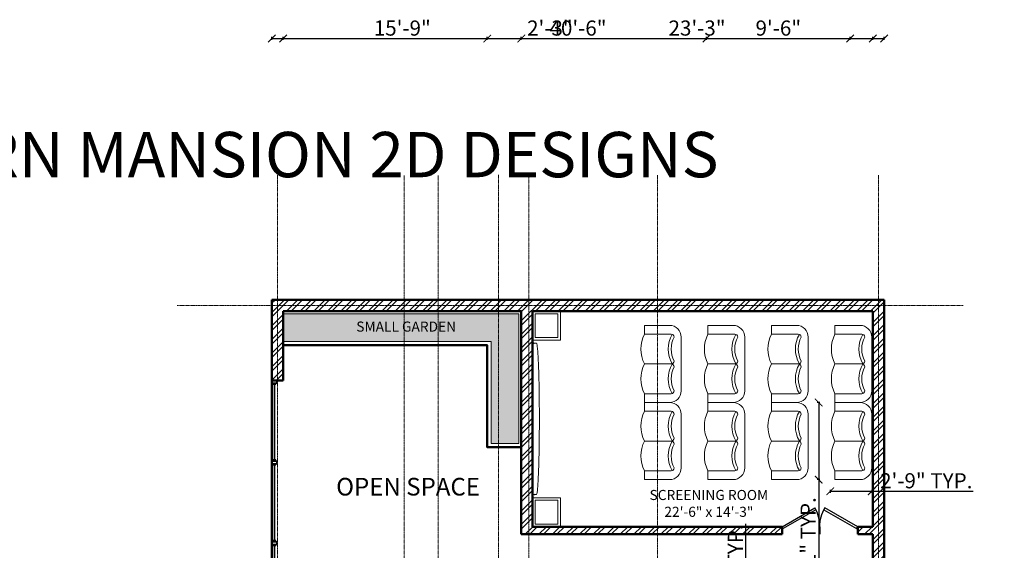
# Model space of a CAD drawing. Units: inches. Extents: x 261 to 2725, y 291 to 1454.
# Tile 25 of 35: x 1043 to 1824, y 1033 to 1454. Entities that reach past the tile are written whole.
import ezdxf

# ---------------------------------------------------------------- set-up
doc = ezdxf.new("R2010")
doc.units = ezdxf.units.IN
doc.linetypes.add('CENTER', pattern=[2, 1.25, -0.25, 0.25, -0.25])
for name, color, linetype, lineweight in [('A-ANNO-DIMS', 136, 'Continuous', 18), ('A-ANNO-TEXT', 7, 'Continuous', 25), ('A-AREA-IDEN', 18, 'Continuous', 18), ('A-DOOR', 160, 'Continuous', 25), ('A-FLOR-FIXT', 145, 'Continuous', 18), ('A-FLOR-HRAL', 132, 'Continuous', 25), ('A-FURN', 30, 'Continuous', 18), ('A-GRID', 251, 'CENTER', 13), ('A-PLNT', 3, 'Continuous', 18), ('A-PLNT-PATT', 3, 'Continuous', 13), ('A-WALL', 222, 'Continuous', 50), ('A-WALL-PATT', 243, 'Continuous', 13)]:
    doc.layers.add(name, color=color, linetype=linetype, lineweight=lineweight)
doc.styles.get("Standard").update_dxf_attribs({"font": 'arial.ttf'})
doc.dimstyles.new('ISO-25', dxfattribs={"dimtxt": 12, "dimasz": 6, "dimexe": 1.25, "dimexo": 0.625, "dimtad": 1, "dimdec": 0, "dimlunit": 3, "dimtxsty": 'Standard', "dimblk": 'ARCHTICK', "dimcen": 2.5, "dimadec": 0, "dimazin": 0, "dimtfac": 1, "dimtdec": 0, "dimtmove": 0, "dimatfit": 3, "dimfxl": 1, "dimfxlon": 1, "dimarcsym": 0})

# ---------------------------------------------------------------- blocks, each defined once
blk = doc.blocks.new('*U10')
for p, q in [((0, 0), (0, -6)), ((30, 0), (30, -6))]:
    blk.add_line(p, q)
blk.add_lwpolyline([(0, 0), (25.98, 15), (26.86, 13.48), (0.88, -1.52)], close=True)
blk.add_arc((0, 0), 30, 0, 30)
blk = doc.blocks.new('A$C16D51D41')
for p, q in [((1.12, 0.69, -343.199), (0.2, 0.69, -343.199)), ((0.15, 0.52, -343.199), (0.15, 0.06, -343.199)), ((0.15, 0.06, -343.199), (0.15, 0.52, -343.199)), ((0.15, 0.52, -343.199), (0.15, 0.06, -343.199)), ((0.66, 0.06, -343.199), (0.66, 0.52, -343.199)), ((0.66, 0.52, -343.199), (0.66, 0.06, -343.199)), ((1.17, 0.52, -343.199), (1.17, 0.06, -343.199)), ((0, 0.49, -343.199), (0, 0.06, -343.199)), ((1.32, 0.06, -343.199), (1.32, 0.49, -343.199)), ((0, 0.06, -343.199), (0.15, 0.06, -343.199)), ((1.32, 0.06, -343.199), (1.17, 0.06, -343.199))]:
    blk.add_line(p, q)
for centre, radius, start, end in [((0.2, 0.49, -343.199), 0.2, 90, 180), ((1.12, 0.49, -343.199), 0.2, 0, 90), ((0.2, 0.52, -343.199), 0.05, 90, 180), ((0.405, 0.965, -343.199), 0.495, 239.4911, 300.5089), ((0.405, 0.965, -343.199), 0.445, 242.5861, 297.4139), ((0.61, 0.52, -343.199), 0.05, 0, 90), ((0.71, 0.52, -343.199), 0.05, 90, 180), ((0.915, 0.965, -343.199), 0.495, 239.4911, 300.5089), ((0.915, 0.965, -343.199), 0.445, 242.5861, 297.4139), ((1.12, 0.52, -343.199), 0.05, 0, 90), ((0.405, 0.572, -343.199), 0.572, 243.519, 296.481), ((0.915, 0.572, -343.199), 0.572, 243.519, 296.481)]:
    blk.add_arc(centre, radius, start, end)
blk = doc.blocks.new('_ArchTick')
at = {"color": 0, "linetype": 'ByBlock', "const_width": 0.15}
blk.add_lwpolyline([(-0.5, -0.5), (0.5, 0.5)], dxfattribs=at)
blk = doc.blocks.new('*D37')
at = {"layer": 'A-ANNO-DIMS', "color": 0, "lineweight": -2, "ltscale": 0.07, "transparency": 16777216}
for p, q in [((1678.14, 1150), (1675.89, 1150)), ((1677.14, 1150), (1677.14, 1088.8)), ((1678.14, 1088.8), (1675.89, 1088.8)), ((1677.14, 1088.8), (1677.14, 871.16))]:
    blk.add_line(p, q, dxfattribs=at)
at = {"layer": 'Defpoints', "color": 0, "ltscale": 0.07, "transparency": 16777216}
for p in [(1686.32, 1150), (1677.14, 1088.8), (1686.32, 1088.8)]:
    blk.add_point(p, dxfattribs=at)
at = {"layer": 'A-ANNO-DIMS', "color": 0, "lineweight": -2, "ltscale": 0.07, "transparency": 16777216, "xscale": 6, "yscale": 6, "zscale": 6}
for p, rotation in [((1677.14, 1150), 90), ((1677.14, 1088.8), 270)]:
    blk.add_blockref('_ArchTick', p, dxfattribs=dict(at, rotation=rotation))
at = {"layer": 'A-ANNO-DIMS', "color": 0, "ltscale": 0.07, "transparency": 16777216, "insert": (1670.31, 976.98), "char_height": 12, "attachment_point": 5, "rotation": 90}
blk.add_mtext('RECLINER SEAT 5\'-1" TYP.', dxfattribs=at)
blk = doc.blocks.new('*D38')
at = {"layer": 'A-ANNO-DIMS', "color": 0, "lineweight": -2, "ltscale": 0.07, "transparency": 16777216}
for p, q in [((1686.32, 1080.62), (1686.32, 1078.37)), ((1686.32, 1079.62), (1719.23, 1079.62)), ((1719.23, 1080.62), (1719.23, 1078.37)), ((1719.23, 1079.62), (1799.83, 1079.62))]:
    blk.add_line(p, q, dxfattribs=at)
at = {"layer": 'Defpoints', "color": 0, "ltscale": 0.07, "transparency": 16777216}
for p in [(1686.32, 1088.8), (1719.23, 1088.8), (1719.23, 1079.62)]:
    blk.add_point(p, dxfattribs=at)
at = {"layer": 'A-ANNO-DIMS', "color": 0, "lineweight": -2, "ltscale": 0.07, "transparency": 16777216, "xscale": 6, "yscale": 6, "zscale": 6, "rotation": 180}
blk.add_blockref('_ArchTick', (1686.32, 1079.62), dxfattribs=at)
at = {"layer": 'A-ANNO-DIMS', "color": 0, "lineweight": -2, "ltscale": 0.07, "transparency": 16777216, "xscale": 6, "yscale": 6, "zscale": 6}
blk.add_blockref('_ArchTick', (1719.23, 1079.62), dxfattribs=at)
at = {"layer": 'A-ANNO-DIMS', "color": 0, "ltscale": 0.07, "transparency": 16777216, "insert": (1762.53, 1086.37), "char_height": 12, "attachment_point": 5}
blk.add_mtext('2\'-9" TYP.', dxfattribs=at)
blk = doc.blocks.new('*D64')
at = {"layer": 'A-ANNO-DIMS', "color": 0, "lineweight": -2, "ltscale": 0.07, "transparency": 16777216}
for p, q in [((1619.28, 973.47), (1619.28, 1053.86)), ((1620.28, 973.47), (1618.03, 973.47)), ((1619.28, 964.47), (1619.28, 973.47)), ((1620.28, 964.47), (1618.03, 964.47))]:
    blk.add_line(p, q, dxfattribs=at)
at = {"layer": 'Defpoints', "color": 0, "ltscale": 0.07, "transparency": 16777216}
for p in [(1619.28, 973.47), (1630.08, 973.47), (1630.08, 964.47)]:
    blk.add_point(p, dxfattribs=at)
at = {"layer": 'A-ANNO-DIMS', "color": 0, "lineweight": -2, "ltscale": 0.07, "transparency": 16777216, "xscale": 6, "yscale": 6, "zscale": 6}
for p, rotation in [((1619.28, 973.47), 90), ((1619.28, 964.47), 270)]:
    blk.add_blockref('_ArchTick', p, dxfattribs=dict(at, rotation=rotation))
at = {"layer": 'A-ANNO-DIMS', "color": 0, "ltscale": 0.07, "transparency": 16777216, "insert": (1612.53, 1016.67), "char_height": 12, "attachment_point": 5, "rotation": 90}
blk.add_mtext('0\'-9" TYP.', dxfattribs=at)
blk = doc.blocks.new('*D85')
at = {"layer": 'A-ANNO-DIMS', "color": 0, "lineweight": -2, "ltscale": 0.07, "transparency": 16777216}
for p, q in [((2600.96, 1222.47), (2603.21, 1222.47)), ((2601.96, 1024.47), (2601.96, 1222.47)), ((2600.96, 1024.47), (2603.21, 1024.47))]:
    blk.add_line(p, q, dxfattribs=at)
at = {"layer": 'Defpoints', "color": 0, "ltscale": 0.07, "transparency": 16777216}
for p in [(946.45, 1222.47), (2601.96, 1222.47), (946.45, 1024.47)]:
    blk.add_point(p, dxfattribs=at)
at = {"layer": 'A-ANNO-DIMS', "color": 0, "lineweight": -2, "ltscale": 0.07, "transparency": 16777216, "xscale": 6, "yscale": 6, "zscale": 6}
for p, rotation in [((2601.96, 1222.47), 90), ((2601.96, 1024.47), 270)]:
    blk.add_blockref('_ArchTick', p, dxfattribs=dict(at, rotation=rotation))
at = {"layer": 'A-ANNO-DIMS', "color": 0, "ltscale": 0.07, "transparency": 16777216, "insert": (2595.21, 1123.47), "char_height": 12, "attachment_point": 5, "rotation": 90}
blk.add_mtext('16\'-6"', dxfattribs=at)
blk = doc.blocks.new('*D102')
at = {"layer": 'A-ANNO-DIMS', "color": 0, "lineweight": -2, "ltscale": 0.07, "transparency": 16777216}
for p, q in [((1243.08, 1437.76), (1243.08, 1440.01)), ((1243.08, 1438.76), (1729.08, 1438.76)), ((1729.08, 1437.76), (1729.08, 1440.01))]:
    blk.add_line(p, q, dxfattribs=at)
at = {"layer": 'Defpoints', "color": 0, "ltscale": 0.07, "transparency": 16777216}
for p in [(1729.08, 1438.76), (1243.08, 1231.47), (1729.08, 1231.47)]:
    blk.add_point(p, dxfattribs=at)
at = {"layer": 'A-ANNO-DIMS', "color": 0, "lineweight": -2, "ltscale": 0.07, "transparency": 16777216, "xscale": 6, "yscale": 6, "zscale": 6, "rotation": 180}
blk.add_blockref('_ArchTick', (1243.08, 1438.76), dxfattribs=at)
at = {"layer": 'A-ANNO-DIMS', "color": 0, "lineweight": -2, "ltscale": 0.07, "transparency": 16777216, "xscale": 6, "yscale": 6, "zscale": 6}
blk.add_blockref('_ArchTick', (1729.08, 1438.76), dxfattribs=at)
at = {"layer": 'A-ANNO-DIMS', "color": 0, "ltscale": 0.07, "transparency": 16777216, "insert": (1486.08, 1445.51), "char_height": 12, "attachment_point": 5}
blk.add_mtext('40\'-6"', dxfattribs=at)
blk = doc.blocks.new('*D103')
at = {"layer": 'A-ANNO-DIMS', "color": 0, "lineweight": -2, "ltscale": 0.07, "transparency": 16777216}
for p, q in [((287.06, 1231.47), (284.81, 1231.47)), ((286.06, 439.47), (286.06, 1231.47)), ((287.06, 439.47), (284.81, 439.47))]:
    blk.add_line(p, q, dxfattribs=at)
at = {"layer": 'Defpoints', "color": 0, "ltscale": 0.07, "transparency": 16777216}
for p in [(286.06, 1231.47), (1243.08, 1231.47), (1243.08, 439.47)]:
    blk.add_point(p, dxfattribs=at)
at = {"layer": 'A-ANNO-DIMS', "color": 0, "lineweight": -2, "ltscale": 0.07, "transparency": 16777216, "xscale": 6, "yscale": 6, "zscale": 6}
for p, rotation in [((286.06, 1231.47), 90), ((286.06, 439.47), 270)]:
    blk.add_blockref('_ArchTick', p, dxfattribs=dict(at, rotation=rotation))
at = {"layer": 'A-ANNO-DIMS', "color": 0, "ltscale": 0.07, "transparency": 16777216, "insert": (279.3, 835.47), "char_height": 12, "attachment_point": 5, "rotation": 90}
blk.add_mtext('66\'-0"', dxfattribs=at)
blk = doc.blocks.new('*D104')
at = {"layer": 'A-ANNO-DIMS', "color": 0, "lineweight": -2, "ltscale": 0.07, "transparency": 16777216}
for p, q in [((1252.08, 1437.76), (1252.08, 1440.01)), ((1252.08, 1438.76), (1441.08, 1438.76)), ((1441.08, 1437.76), (1441.08, 1440.01))]:
    blk.add_line(p, q, dxfattribs=at)
at = {"layer": 'Defpoints', "color": 0, "ltscale": 0.07, "transparency": 16777216}
for p in [(1441.08, 1438.76), (1252.08, 1222.47), (1441.08, 1222.47)]:
    blk.add_point(p, dxfattribs=at)
at = {"layer": 'A-ANNO-DIMS', "color": 0, "lineweight": -2, "ltscale": 0.07, "transparency": 16777216, "xscale": 6, "yscale": 6, "zscale": 6, "rotation": 180}
blk.add_blockref('_ArchTick', (1252.08, 1438.76), dxfattribs=at)
at = {"layer": 'A-ANNO-DIMS', "color": 0, "lineweight": -2, "ltscale": 0.07, "transparency": 16777216, "xscale": 6, "yscale": 6, "zscale": 6}
blk.add_blockref('_ArchTick', (1441.08, 1438.76), dxfattribs=at)
at = {"layer": 'A-ANNO-DIMS', "color": 0, "ltscale": 0.07, "transparency": 16777216, "insert": (1346.58, 1445.51), "char_height": 12, "attachment_point": 5}
blk.add_mtext('15\'-9"', dxfattribs=at)
blk = doc.blocks.new('*D105')
at = {"layer": 'A-ANNO-DIMS', "color": 0, "lineweight": -2, "ltscale": 0.07, "transparency": 16777216}
for p, q in [((1441.08, 1437.76), (1441.08, 1440.01)), ((1441.08, 1438.76), (1720.08, 1438.76)), ((1720.08, 1437.76), (1720.08, 1440.01))]:
    blk.add_line(p, q, dxfattribs=at)
at = {"layer": 'Defpoints', "color": 0, "ltscale": 0.07, "transparency": 16777216}
for p in [(1720.08, 1438.76), (1441.08, 1222.47), (1720.08, 1222.47)]:
    blk.add_point(p, dxfattribs=at)
at = {"layer": 'A-ANNO-DIMS', "color": 0, "lineweight": -2, "ltscale": 0.07, "transparency": 16777216, "xscale": 6, "yscale": 6, "zscale": 6, "rotation": 180}
blk.add_blockref('_ArchTick', (1441.08, 1438.76), dxfattribs=at)
at = {"layer": 'A-ANNO-DIMS', "color": 0, "lineweight": -2, "ltscale": 0.07, "transparency": 16777216, "xscale": 6, "yscale": 6, "zscale": 6}
blk.add_blockref('_ArchTick', (1720.08, 1438.76), dxfattribs=at)
at = {"layer": 'A-ANNO-DIMS', "color": 0, "ltscale": 0.07, "transparency": 16777216, "insert": (1580.58, 1445.52), "char_height": 12, "attachment_point": 5}
blk.add_mtext('23\'-3"', dxfattribs=at)
blk = doc.blocks.new('*D110')
at = {"layer": 'A-ANNO-DIMS', "color": 0, "lineweight": -2, "ltscale": 0.07, "transparency": 16777216}
for p, q in [((287.06, 1222.47), (284.81, 1222.47)), ((286.06, 964.47), (286.06, 1222.47)), ((287.06, 964.47), (284.81, 964.47))]:
    blk.add_line(p, q, dxfattribs=at)
at = {"layer": 'Defpoints', "color": 0, "ltscale": 0.07, "transparency": 16777216}
for p in [(286.06, 1222.47), (1252.08, 1222.47), (1252.08, 964.47)]:
    blk.add_point(p, dxfattribs=at)
at = {"layer": 'A-ANNO-DIMS', "color": 0, "lineweight": -2, "ltscale": 0.07, "transparency": 16777216, "xscale": 6, "yscale": 6, "zscale": 6}
for p, rotation in [((286.06, 1222.47), 90), ((286.06, 964.47), 270)]:
    blk.add_blockref('_ArchTick', p, dxfattribs=dict(at, rotation=rotation))
at = {"layer": 'A-ANNO-DIMS', "color": 0, "ltscale": 0.07, "transparency": 16777216, "insert": (279.3, 1093.47), "char_height": 12, "attachment_point": 5, "rotation": 90}
blk.add_mtext('21\'-6"', dxfattribs=at)
blk = doc.blocks.new('*D115')
at = {"layer": 'A-ANNO-DIMS', "color": 0, "lineweight": -2, "ltscale": 0.07, "transparency": 16777216}
for p, q in [((2600.96, 1222.47), (2603.21, 1222.47)), ((2601.96, 964.47), (2601.96, 1222.47)), ((2600.96, 964.47), (2603.21, 964.47))]:
    blk.add_line(p, q, dxfattribs=at)
at = {"layer": 'Defpoints', "color": 0, "ltscale": 0.07, "transparency": 16777216}
for p in [(1720.08, 1222.47), (2601.96, 1222.47), (1720.08, 964.47)]:
    blk.add_point(p, dxfattribs=at)
at = {"layer": 'A-ANNO-DIMS', "color": 0, "lineweight": -2, "ltscale": 0.07, "transparency": 16777216, "xscale": 6, "yscale": 6, "zscale": 6}
for p, rotation in [((2601.96, 1222.47), 90), ((2601.96, 964.47), 270)]:
    blk.add_blockref('_ArchTick', p, dxfattribs=dict(at, rotation=rotation))
at = {"layer": 'A-ANNO-DIMS', "color": 0, "ltscale": 0.07, "transparency": 16777216, "insert": (2595.21, 1093.47), "char_height": 12, "attachment_point": 5, "rotation": 90}
blk.add_mtext('21\'-6"', dxfattribs=at)
blk = doc.blocks.new('*D117')
at = {"layer": 'A-ANNO-DIMS', "color": 0, "lineweight": -2, "ltscale": 0.07, "transparency": 16777216}
for p, q in [((1588.08, 1437.76), (1588.08, 1440.01)), ((1588.08, 1438.76), (1702.08, 1438.76)), ((1702.08, 1437.76), (1702.08, 1440.01))]:
    blk.add_line(p, q, dxfattribs=at)
at = {"layer": 'Defpoints', "color": 0, "ltscale": 0.07, "transparency": 16777216}
for p in [(1702.08, 1438.76), (1588.08, 559.47), (1702.08, 559.47)]:
    blk.add_point(p, dxfattribs=at)
at = {"layer": 'A-ANNO-DIMS', "color": 0, "lineweight": -2, "ltscale": 0.07, "transparency": 16777216, "xscale": 6, "yscale": 6, "zscale": 6, "rotation": 180}
blk.add_blockref('_ArchTick', (1588.08, 1438.76), dxfattribs=at)
at = {"layer": 'A-ANNO-DIMS', "color": 0, "lineweight": -2, "ltscale": 0.07, "transparency": 16777216, "xscale": 6, "yscale": 6, "zscale": 6}
blk.add_blockref('_ArchTick', (1702.08, 1438.76), dxfattribs=at)
at = {"layer": 'A-ANNO-DIMS', "color": 0, "ltscale": 0.07, "transparency": 16777216, "insert": (1645.08, 1445.51), "char_height": 12, "attachment_point": 5}
blk.add_mtext('9\'-6"', dxfattribs=at)
blk = doc.blocks.new('*D118')
at = {"layer": 'A-ANNO-DIMS', "color": 0, "lineweight": -2, "ltscale": 0.07, "transparency": 16777216}
for p, q in [((287.06, 1222.47), (284.81, 1222.47)), ((286.06, 1222.47), (286.06, 1195.47)), ((287.06, 1195.47), (284.81, 1195.47)), ((286.06, 1195.47), (286.06, 1156.11))]:
    blk.add_line(p, q, dxfattribs=at)
at = {"layer": 'Defpoints', "color": 0, "ltscale": 0.07, "transparency": 16777216}
for p in [(1252.08, 1222.47), (286.06, 1195.47), (1252.08, 1195.47)]:
    blk.add_point(p, dxfattribs=at)
at = {"layer": 'A-ANNO-DIMS', "color": 0, "lineweight": -2, "ltscale": 0.07, "transparency": 16777216, "xscale": 6, "yscale": 6, "zscale": 6}
for p, rotation in [((286.06, 1222.47), 90), ((286.06, 1195.47), 270)]:
    blk.add_blockref('_ArchTick', p, dxfattribs=dict(at, rotation=rotation))
at = {"layer": 'A-ANNO-DIMS', "color": 0, "ltscale": 0.07, "transparency": 16777216, "insert": (279.3, 1172.79), "char_height": 12, "attachment_point": 5, "rotation": 90}
blk.add_mtext('2\'-3"', dxfattribs=at)
blk = doc.blocks.new('*D119')
at = {"layer": 'A-ANNO-DIMS', "color": 0, "lineweight": -2, "ltscale": 0.07, "transparency": 16777216}
for p, q in [((1414.08, 1437.76), (1414.08, 1440.01)), ((1414.08, 1438.76), (1441.08, 1438.76)), ((1441.08, 1437.76), (1441.08, 1440.01)), ((1441.08, 1438.76), (1480.43, 1438.76))]:
    blk.add_line(p, q, dxfattribs=at)
at = {"layer": 'Defpoints', "color": 0, "ltscale": 0.07, "transparency": 16777216}
for p in [(1441.08, 1438.76), (1414.08, 1114.47), (1441.08, 1114.47)]:
    blk.add_point(p, dxfattribs=at)
at = {"layer": 'A-ANNO-DIMS', "color": 0, "lineweight": -2, "ltscale": 0.07, "transparency": 16777216, "xscale": 6, "yscale": 6, "zscale": 6, "rotation": 180}
blk.add_blockref('_ArchTick', (1414.08, 1438.76), dxfattribs=at)
at = {"layer": 'A-ANNO-DIMS', "color": 0, "lineweight": -2, "ltscale": 0.07, "transparency": 16777216, "xscale": 6, "yscale": 6, "zscale": 6}
blk.add_blockref('_ArchTick', (1441.08, 1438.76), dxfattribs=at)
at = {"layer": 'A-ANNO-DIMS', "color": 0, "ltscale": 0.07, "transparency": 16777216, "insert": (1463.76, 1445.52), "char_height": 12, "attachment_point": 5}
blk.add_mtext('2\'-3"', dxfattribs=at)
blk = doc.blocks.new('*D123')
at = {"layer": 'A-ANNO-DIMS', "color": 0, "lineweight": -2, "ltscale": 0.07, "transparency": 16777216}
for p, q in [((287.06, 1054.85), (284.81, 1054.85)), ((286.06, 439.47), (286.06, 1054.85)), ((287.06, 439.47), (284.81, 439.47))]:
    blk.add_line(p, q, dxfattribs=at)
at = {"layer": 'Defpoints', "color": 0, "ltscale": 0.07, "transparency": 16777216}
for p in [(286.06, 1054.85), (2007.71, 1054.85), (2007.71, 439.47)]:
    blk.add_point(p, dxfattribs=at)
at = {"layer": 'A-ANNO-DIMS', "color": 0, "lineweight": -2, "ltscale": 0.07, "transparency": 16777216, "xscale": 6, "yscale": 6, "zscale": 6}
for p, rotation in [((286.06, 1054.85), 90), ((286.06, 439.47), 270)]:
    blk.add_blockref('_ArchTick', p, dxfattribs=dict(at, rotation=rotation))
at = {"layer": 'A-ANNO-DIMS', "color": 0, "ltscale": 0.07, "transparency": 16777216, "insert": (279.22, 747.16), "char_height": 12, "attachment_point": 5, "rotation": 90}
blk.add_mtext('51\'-3 1/2"', dxfattribs=at)

msp = doc.modelspace()

# ---------------------------------------------------------------- hatches: boundary and pattern name
at = {"layer": 'A-PLNT-PATT'}
h = msp.add_hatch(dxfattribs=at)
h.set_pattern_fill('GRASS', color=256, scale=0.7)
h.paths.add_polyline_path([(658.45, 427.47), (433.45, 427.47), (433.45, 415.47), (658.45, 415.47)])
h.paths.add_polyline_path([(670.45, 421.47), (664.45, 421.47), (664.45, 415.47), (670.45, 415.47)])
h.paths.add_polyline_path([(784.45, 421.47), (778.45, 421.47), (778.45, 415.47), (784.45, 415.47)])
h.paths.add_polyline_path([(991.45, 427.47), (790.45, 427.47), (790.45, 415.47), (991.45, 415.47)])
h.paths.add_polyline_path([(1439.08, 1220.47), (1252.08, 1220.47), (1252.08, 1198.47), (1417.08, 1198.47), (1417.08, 1117.47), (1439.08, 1117.47)])
h.paths.add_polyline_path([(2304.71, 1045.85), (2016.71, 1045.85), (2016.71, 805.87), (2304.71, 805.87)])
h.paths.add_polyline_path([(1267.21, 1201.68), (1431.59, 1201.68), (1431.59, 1218.76), (1267.21, 1218.76)], flags=24)
h.paths.add_polyline_path([(2089.2, 883.04), (2242.64, 883.04), (2242.64, 936.27), (2089.2, 936.27)], flags=24)
at = {"layer": 'A-WALL-PATT'}
h = msp.add_hatch(dxfattribs=at)
h.set_pattern_fill('ANSI32', color=256, scale=0.8)
h.paths.add_polyline_path([(478.45, 685.47), (580.45, 685.47), (580.45, 691.47), (577.45, 691.47), (577.45, 694.47), (571.45, 694.47), (571.45, 691.47), (478.45, 691.47), (478.45, 721.47), (469.45, 721.47), (469.45, 508.47), (538.45, 508.47), (538.45, 517.47), (478.45, 517.47)])
h.paths.add_polyline_path([(694.45, 517.47), (676.45, 517.47), (676.45, 646.47), (670.45, 646.47), (670.45, 517.47), (610.45, 517.47), (610.45, 508.47), (694.45, 508.47)])
h.paths.add_polyline_path([(676.45, 784.47), (478.45, 784.47), (478.45, 844.47), (469.45, 844.47), (469.45, 745.47), (478.45, 745.47), (478.45, 775.47), (571.45, 775.47), (571.45, 724.47), (577.45, 724.47), (577.45, 775.47), (670.45, 775.47), (670.45, 691.47), (610.45, 691.47), (610.45, 685.47), (670.45, 685.47), (670.45, 682.47), (676.45, 682.47)])
h.paths.add_polyline_path([(955.45, 880.47), (946.45, 880.47), (946.45, 808.47), (778.45, 808.47), (778.45, 799.47), (946.45, 799.47), (946.45, 517.47), (898.45, 517.47), (898.45, 508.47), (955.45, 508.47)])
h.paths.add_polyline_path([(778.45, 598.47), (772.45, 598.47), (772.45, 517.47), (754.45, 517.47), (754.45, 508.47), (826.45, 508.47), (826.45, 517.47), (778.45, 517.47)])
h.paths.add_polyline_path([(955.45, 1090.47), (946.45, 1090.47), (946.45, 1030.47), (817.45, 1030.47), (817.45, 1024.47), (946.45, 1024.47), (946.45, 952.47), (955.45, 952.47)])
h.paths.add_polyline_path([(955.45, 1231.47), (730.45, 1231.47), (730.45, 1222.47), (772.45, 1222.47), (772.45, 1096.47), (766.45, 1096.47), (766.45, 1090.47), (772.45, 1090.47), (772.45, 1006.47), (712.45, 1006.47), (712.45, 1000.47), (778.45, 1000.47), (778.45, 1024.47), (781.45, 1024.47), (781.45, 1030.47), (778.45, 1030.47), (778.45, 1222.47), (946.45, 1222.47), (946.45, 1162.47), (955.45, 1162.47)])
h.paths.add_polyline_path([(694.45, 1231.47), (619.45, 1231.47), (619.45, 1222.47), (646.45, 1222.47), (646.45, 1039.47), (652.45, 1039.47), (652.45, 1090.47), (736.45, 1090.47), (736.45, 1096.47), (652.45, 1096.47), (652.45, 1222.47), (694.45, 1222.47)])
h.paths.add_polyline_path([(571.45, 1231.47), (469.45, 1231.47), (469.45, 1099.47), (478.45, 1099.47), (478.45, 1144.47), (544.45, 1144.47), (544.45, 1153.47), (538.45, 1153.47), (538.45, 1150.47), (478.45, 1150.47), (478.45, 1222.47), (538.45, 1222.47), (538.45, 1183.47), (544.45, 1183.47), (544.45, 1222.47), (571.45, 1222.47)])
h.paths.add_polyline_path([(538.45, 1006.47), (478.45, 1006.47), (478.45, 1051.47), (469.45, 1051.47), (469.45, 940.47), (478.45, 940.47), (478.45, 1000.47), (538.45, 1000.47)])
h.paths.add_polyline_path([(652.45, 1006.47), (652.45, 1009.47), (646.45, 1009.47), (646.45, 1006.47), (586.45, 1006.47), (586.45, 1000.47), (652.45, 1000.47)])
h.paths.add_polyline_path([(1288.08, 973.47), (1243.08, 973.47), (1243.08, 920.97), (1252.08, 920.97), (1252.08, 964.47), (1288.08, 964.47)], flags=17)
h.paths.add_polyline_path([(1402.08, 805.47), (1252.08, 805.47), (1252.08, 848.97), (1243.08, 848.97), (1243.08, 757.47), (1252.08, 757.47), (1252.08, 799.47), (1294.08, 799.47), (1372.08, 799.47), (1372.08, 779.47), (1372.08, 715.47), (1378.08, 715.47), (1378.08, 799.47), (1402.08, 799.47)])
h.paths.add_polyline_path([(1252.08, 721.47), (1243.08, 721.47), (1243.08, 439.47), (1729.08, 439.47), (1729.08, 709.47), (1720.08, 709.47), (1720.08, 679.47), (1582.08, 679.47), (1582.08, 670.47), (1588.08, 670.47), (1588.08, 673.47), (1720.08, 673.47), (1720.08, 559.47), (1690.08, 559.47), (1690.08, 550.47), (1720.08, 550.47), (1720.08, 448.47), (1252.08, 448.47), (1252.08, 496.47), (1312.08, 496.47), (1312.08, 505.47), (1252.08, 505.47), (1252.08, 673.47), (1405.08, 673.47), (1405.08, 679.47), (1378.08, 679.47), (1378.08, 685.47), (1372.08, 685.47), (1372.08, 679.47), (1252.08, 679.47)])
h.paths.add_polyline_path([(1450.08, 550.47), (1480.08, 550.47), (1480.08, 559.47), (1450.08, 559.47), (1450.08, 679.47), (1441.08, 679.47), (1441.08, 673.47), (1444.08, 673.47), (1444.08, 505.47), (1384.08, 505.47), (1384.08, 496.47), (1450.08, 496.47)], flags=17)
h.paths.add_polyline_path([(1618.08, 559.47), (1588.08, 559.47), (1588.08, 634.47), (1582.08, 634.47), (1582.08, 559.47), (1552.08, 559.47), (1552.08, 550.47), (1618.08, 550.47)], flags=17)
h.paths.add_polyline_path([(1564.08, 964.47), (1630.08, 964.47), (1630.08, 973.47), (1477.08, 973.47), (1477.08, 964.47), (1558.08, 964.47), (1558.08, 926.22), (1558.08, 887.97), (1486.08, 887.97), (1486.08, 881.97), (1558.08, 881.97), (1558.08, 805.47), (1450.08, 805.47), (1450.08, 845.97), (1444.08, 845.97), (1444.08, 805.47), (1438.08, 805.47), (1438.08, 799.47), (1564.08, 799.47)], flags=17)
h.paths.add_polyline_path([(1453.08, 973.47), (1408.08, 973.47), (1408.08, 964.47), (1444.08, 964.47), (1444.08, 881.97), (1450.08, 881.97), (1456.08, 881.97), (1456.08, 887.97), (1450.08, 887.97), (1450.08, 964.47), (1453.08, 964.47)], flags=17)
h.paths.add_polyline_path([(1729.08, 1231.47), (1243.08, 1231.47), (1243.08, 1167.47), (1252.08, 1167.47), (1252.08, 1222.47), (1441.08, 1222.47), (1441.08, 1045.47), (1648.08, 1045.47), (1648.08, 1051.47), (1450.08, 1051.47), (1450.08, 1074.47), (1450.08, 1222.47), (1472.08, 1222.47), (1720.08, 1222.47), (1720.08, 1051.47), (1708.08, 1051.47), (1708.08, 1045.47), (1720.08, 1045.47), (1720.08, 973.47), (1702.08, 973.47), (1702.08, 964.47), (1720.08, 964.47), (1720.08, 769.47), (1729.08, 769.47)])
h.paths.add_polyline_path([(2493.71, 1054.85), (2007.71, 1054.85), (2007.71, 439.47), (2214.67, 439.47), (2214.67, 496.47), (2493.71, 496.47)])
h.paths.add_polyline_path([(2016.71, 1045.85), (2304.71, 1045.85), (2304.71, 841.47), (2310.71, 841.47), (2310.71, 1045.85), (2484.71, 1045.85), (2484.71, 805.47), (2310.71, 805.47), (2310.71, 811.47), (2304.71, 811.47), (2304.71, 799.47), (2484.71, 799.47), (2484.71, 679.47), (2304.71, 679.47), (2304.71, 673.47), (2484.71, 673.47), (2484.71, 505.47), (2208.67, 505.47), (2208.67, 448.47), (2016.71, 448.47), (2016.71, 799.47), (2304.71, 799.47), (2304.71, 805.47), (2016.71, 805.47)], flags=16)

# ---------------------------------------------------------------- linework, layer by layer
at = {"layer": 'A-FLOR-FIXT'}
for points in [[(1450.08, 1222.47), (1472.08, 1222.47), (1472.08, 1199.47), (1450.08, 1199.47)], [(1452.08, 1220.47), (1470.08, 1220.47), (1470.08, 1201.47), (1452.08, 1201.47)], [(1450.08, 1051.47), (1472.08, 1051.47), (1472.08, 1074.47), (1450.08, 1074.47)], [(1452.08, 1053.47), (1470.08, 1053.47), (1470.08, 1072.47), (1452.08, 1072.47)]]:
    msp.add_lwpolyline(points, close=True, dxfattribs=at)
msp.add_rational_spline([(1453.08, 1076.97), (1455.41, 1076.97), (1455.41, 1136.97), (1455.41, 1196.97), (1453.08, 1196.97), (1451.58, 1196.97), (1450.08, 1196.97), (1450.08, 1136.97), (1450.08, 1076.97), (1451.58, 1076.97), (1453.08, 1076.97)], [1, 0.707106781187, 1, 0.707106781187, 1, 1, 1, 1, 1, 1, 1], degree=2, knots=[0, 0, 0, 1.570796, 1.570796, 3.141593, 3.141593, 4.141593, 4.141593, 5.141593, 5.141593, 6.141593, 6.141593, 6.141593], dxfattribs=at)
at = {"layer": 'A-FLOR-HRAL'}
for points in [[(1243.08, 1165.47), (1247.08, 1165.47), (1247.08, 1167.47), (1243.08, 1167.47)], [(1243.83, 1164.47), (1246.33, 1164.47), (1246.33, 1165.47), (1243.83, 1165.47)], [(1244.83, 1104.47), (1245.33, 1104.47), (1245.33, 1164.47), (1244.83, 1164.47)], [(1243.08, 1101.47), (1247.08, 1101.47), (1247.08, 1103.47), (1243.08, 1103.47)], [(1243.83, 1103.47), (1246.33, 1103.47), (1246.33, 1104.47), (1243.83, 1104.47)], [(1243.83, 1100.47), (1246.33, 1100.47), (1246.33, 1101.47), (1243.83, 1101.47)], [(1244.83, 1040.47), (1245.33, 1040.47), (1245.33, 1100.47), (1244.83, 1100.47)], [(1243.83, 1039.47), (1246.33, 1039.47), (1246.33, 1040.47), (1243.83, 1040.47)], [(1243.08, 1037.47), (1247.08, 1037.47), (1247.08, 1039.47), (1243.08, 1039.47)], [(1243.83, 1036.47), (1246.33, 1036.47), (1246.33, 1037.47), (1243.83, 1037.47)], [(1244.83, 976.47), (1245.33, 976.47), (1245.33, 1036.47), (1244.83, 1036.47)]]:
    msp.add_lwpolyline(points, close=True, dxfattribs=at)
at = {"layer": 'A-GRID', "ltscale": 0.5}
for p, q in [((1247.58, 1330.47), (1247.58, 416.47)), ((1348.08, 1330.18), (1348.08, 416.18)), ((1375.08, 1330.18), (1375.08, 416.18)), ((1423.08, 1330.51), (1423.08, 416.51)), ((1447.08, 1330.51), (1447.08, 416.51)), ((1549.08, 1330.47), (1549.08, 416.47)), ((1724.58, 1330.47), (1724.58, 416.47)), ((1167.93, 1226.97), (1791.93, 1226.97))]:
    msp.add_line(p, q, dxfattribs=at)
at = {"layer": 'A-PLNT'}
for points in [[(1252.08, 1220.47), (1439.08, 1220.47), (1439.08, 1117.47)], [(1252.08, 1198.47), (1417.08, 1198.47), (1417.08, 1117.47), (1439.08, 1117.47)]]:
    msp.add_lwpolyline(points, dxfattribs=at)
at = {"layer": 'A-WALL'}
for p, q in [((1243.08, 1231.47), (1729.08, 1231.47)), ((1243.08, 1231.47), (1243.08, 920.97)), ((1729.08, 1231.47), (1729.08, 769.47)), ((1252.08, 1222.47), (1252.08, 1167.47)), ((1450.08, 1222.47), (1450.08, 1051.47)), ((1450.08, 1222.47), (1720.08, 1222.47)), ((1720.08, 1222.47), (1720.08, 1051.47)), ((1252.08, 1167.47), (1243.08, 1167.47)), ((1648.08, 1051.47), (1450.08, 1051.47)), ((1648.08, 1045.47), (1648.08, 1051.47)), ((1720.08, 1051.47), (1708.08, 1051.47)), ((1708.08, 1045.47), (1708.08, 1051.47)), ((1648.08, 1045.47), (1441.08, 1045.47)), ((1720.08, 1045.47), (1708.08, 1045.47)), ((1720.08, 1045.47), (1720.08, 973.47))]:
    msp.add_line(p, q, dxfattribs=at)
for points in [[(1252.08, 1222.47), (1441.08, 1222.47), (1441.08, 1045.47)], [(1252.08, 1195.47), (1414.08, 1195.47), (1414.08, 1114.47), (1441.08, 1114.47)]]:
    msp.add_lwpolyline(points, dxfattribs=at)

# ---------------------------------------------------------------- block references
at = {"layer": 'A-DOOR'}
msp.add_blockref('*U10', (1648.08, 1051.47), dxfattribs=at)
at = {"layer": 'A-DOOR', "xscale": -1}
msp.add_blockref('*U10', (1708.08, 1051.47), dxfattribs=at)
at = {"layer": 'A-FURN', "xscale": 46.35909022542807, "yscale": 46.35909022542807, "zscale": 46.35909022542807, "rotation": 270}
for p in [(1535.97, 1211.19, 15910.39), (1586.4, 1211.19, 15910.39), (1636.82, 1211.19, 15910.39), (1687.24, 1211.19, 15910.39), (1535.97, 1150, 15910.39), (1586.4, 1150, 15910.39), (1636.82, 1150, 15910.39), (1687.24, 1150, 15910.39)]:
    msp.add_blockref('A$C16D51D41', p, dxfattribs=at)

# ---------------------------------------------------------------- texts
at = {"layer": 'A-ANNO-TEXT', "insert": (872, 1364.68), "char_height": 36, "attachment_point": 1}
msp.add_mtext_dynamic_manual_height_columns('{\\fTimes New Roman|b1|i0|c0|p18;\\T1.4;MODERN MANSION 2D DESIGNS}', width=1067.3388, gutter_width=12.5, heights=[0], dxfattribs=at)
at = {"layer": 'A-AREA-IDEN', "attachment_point": 1}
for s, width, insert, char_height in [('\\pxqc,t10;{\\fTimes New Roman|b0|i0|c0|p18;\\T2.2;SMALL GARDEN}', 166.064, (1266.65, 1214.23), 8), ('\\pxqc;{\\fTimes New Roman|b0|i0|c0|p18;OPEN SPACE}', 141.595, (1280.39, 1090.21), 14), ('\\pxqc;{\\fTimes New Roman|b0|i0|c0|p18;SCREENING ROOM\\P22\'-6" x 14\'-3"}', 112.0362, (1533.95, 1080.63), 8)]:
    msp.add_mtext_dynamic_manual_height_columns(s, width=width, gutter_width=12.5, heights=[0], dxfattribs=dict(at, insert=insert, char_height=char_height))

# ---------------------------------------------------------------- dimensions: what is measured, and where the dimension line sits
at = {"layer": 'A-ANNO-DIMS', "ltscale": 0.07}
for base, p1, p2, picture, middle in [((1729.08, 1438.76), (1243.08, 1231.47), (1729.08, 1231.47), '*D102', (1486.08, 1445.51)), ((1441.08, 1438.76), (1252.08, 1222.47), (1441.08, 1222.47), '*D104', (1346.58, 1445.51)), ((1441.08, 1438.76), (1414.08, 1114.47), (1441.08, 1114.47), '*D119', (1463.76, 1445.52)), ((1720.08, 1438.76), (1441.08, 1222.47), (1720.08, 1222.47), '*D105', (1580.58, 1445.52)), ((1702.08, 1438.76), (1588.08, 559.47), (1702.08, 559.47), '*D117', (1645.08, 1445.51))]:
    dim = msp.add_linear_dim(base=base, p1=p1, p2=p2, dimstyle='ISO-25', override={"dimdec": 1, "dimlfac": 1, "dimrnd": 0, "dimzin": 1, "dimdsep": 46, "dimlunit": 4, "dimfrac": 2}, dxfattribs=at)
    dim.commit()
    dim.dimension.update_dxf_attribs({"geometry": picture, "text_midpoint": middle})
for base, p1, p2, picture, middle in [((286.06, 1231.47), (1243.08, 439.47), (1243.08, 1231.47), '*D103', (279.3, 835.47)), ((286.06, 1195.47), (1252.08, 1222.47), (1252.08, 1195.47), '*D118', (279.3, 1172.79)), ((286.06, 1222.47), (1252.08, 964.47), (1252.08, 1222.47), '*D110', (279.3, 1093.47)), ((2601.96, 1222.47), (946.45, 1024.47), (946.45, 1222.47), '*D85', (2595.21, 1123.47)), ((2601.96, 1222.47), (1720.08, 964.47), (1720.08, 1222.47), '*D115', (2595.21, 1093.47)), ((286.06, 1054.85), (2007.71, 439.47), (2007.71, 1054.85), '*D123', (279.22, 747.16))]:
    dim = msp.add_linear_dim(base=base, p1=p1, p2=p2, angle=90, dimstyle='ISO-25', override={"dimdec": 1, "dimlfac": 1, "dimrnd": 0, "dimzin": 1, "dimdsep": 46, "dimlunit": 4, "dimfrac": 2}, dxfattribs=at)
    dim.commit()
    dim.dimension.update_dxf_attribs({"geometry": picture, "text_midpoint": middle})
for base, p1, p2, angle, text, picture, middle in [((1677.14, 1088.8), (1686.32, 1150), (1686.32, 1088.8), 270, 'RECLINER SEAT <> TYP.', '*D37', (1670.31, 976.98)), ((1619.28, 973.47), (1630.08, 964.47), (1630.08, 973.47), 90, '<> TYP.', '*D64', (1612.53, 1016.67))]:
    dim = msp.add_linear_dim(base=base, p1=p1, p2=p2, angle=angle, text=text, dimstyle='ISO-25', override={"dimdec": 1, "dimrnd": 0, "dimzin": 1, "dimlunit": 4, "dimfrac": 2}, dxfattribs=at)
    dim.commit()
    dim.dimension.update_dxf_attribs({"geometry": picture, "text_midpoint": middle})
dim = msp.add_linear_dim(base=(1719.23, 1079.62), p1=(1686.32, 1088.8), p2=(1719.23, 1088.8), text='<> TYP.', dimstyle='ISO-25', override={"dimdec": 1, "dimrnd": 0, "dimzin": 1, "dimlunit": 4, "dimfrac": 2}, dxfattribs=at)
dim.commit()
dim.dimension.update_dxf_attribs({"geometry": '*D38', "text_midpoint": (1762.53, 1086.37)})

doc.saveas('drawing.dxf')
